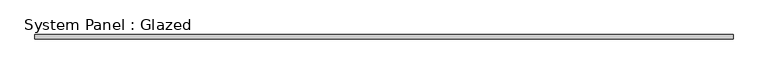
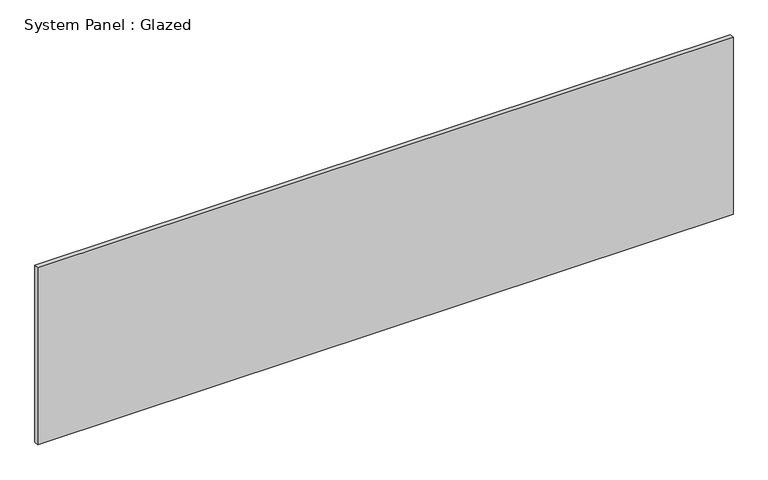
"""IFC4 building model written with IfcOpenShell, lengths in millimetres: plate geometry, System Panel : Glazed."""

from ifc_helpers import new_model, si_unit, origin, origin_with_axes, place, context, project, spatial, polyline, outline, extrude, source, transform, mapped, element, save


def system_panel_glazed_b77e27d4(model_context):
    return source(origin(), model_context, "Body", "SweptSolid", [
        extrude(outline(polyline([(1955.8, 19.05), (-1955.8, 19.05), (-1955.8, 44.45), (1955.8, 44.45), (1955.8, 19.05)])), origin_with_axes(), (0.0, 0.0, 1.0), 1052.0553742),
    ])


if __name__ == "__main__":
    model = new_model("IFC4")
    model_context = context("Model", 3, world=origin())
    ifc_project = project(units=[si_unit("LENGTHUNIT", "METRE", prefix="MILLI")], contexts=[model_context])
    site = spatial("IfcSite", under=ifc_project)
    building = spatial("IfcBuilding", under=site)
    placement = place(None, origin())
    system_panel_glazed_shape = system_panel_glazed_b77e27d4(model_context)
    element("IfcPlate", 1, ObjectType="System Panel : Glazed", at=placement, inside=building, context=model_context, shape_type="MappedRepresentation", body=[
        mapped(system_panel_glazed_shape, transform((0.0, 0.0, 0.0), x_axis=(1.0, 0.0, 0.0), y_axis=(0.0, 1.0, 0.0), z_axis=(0.0, 0.0, 1.0))),
    ])
    save(model, "model.ifc")

# Revit data of these elements
# Type "System Panel : Glazed"
#   Construction Type Id = "GSP4R"
#   Analytic Construction = "1/8 in Pilkington single glazing"
#   Visual Light Transmittance = 0.9
#   Solar Heat Gain Coefficient = 0.86
#   Heat Transfer Coefficient (U) = 1.18115 BTU/(h·ft²·°F)
#   Define Thermal Properties by = 1
# Element 1 (IfcPlate, "System Panel : Glazed")
#   Materials on its faces: "Glass"
# Materials
#   "Glass": class "Glass", colour RGB 0 128 192, transparency 0.75, Description = "Soda Lime Glass", Cost = 0
